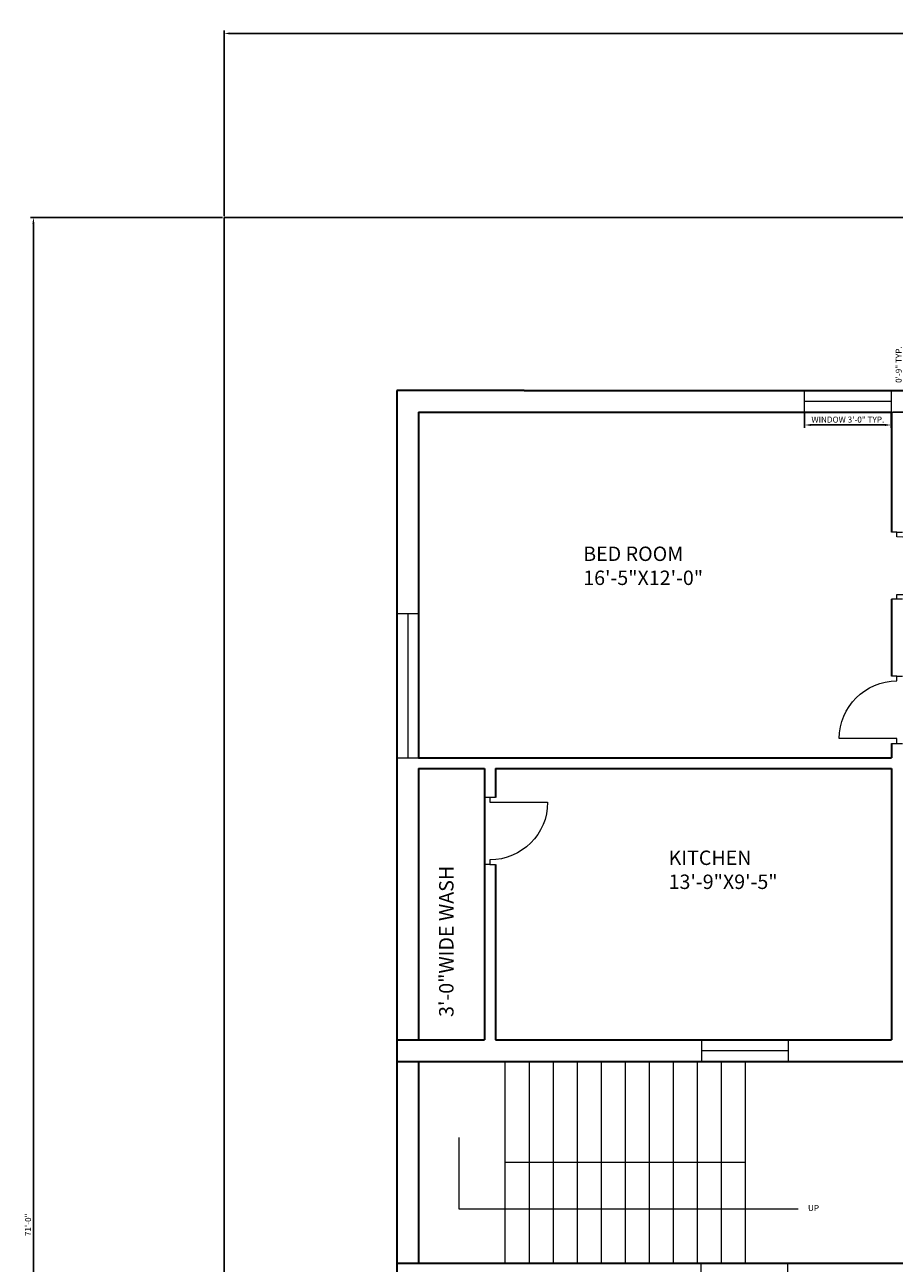
# Model space of a CAD drawing. Units: inches. Extents: x 3257 to 4085, y -12 to 956.
# Tile 4 of 6: x 3257 to 3619, y 441 to 956. Entities that reach past the tile are written whole.
import ezdxf

# ---------------------------------------------------------------- set-up
doc = ezdxf.new("R2010")
doc.units = ezdxf.units.IN
for name, color, linetype, lineweight in [('A-ANNO-DIMS', 2, 'Continuous', 18), ('A-ANNO-TEXT', 7, 'Continuous', 18), ('A-AREA-IDEN', 7, 'Continuous', 18), ('A-DOOR', 3, 'Continuous', 18), ('A-FLOR-STRS', 7, 'Continuous', 18), ('A-GLAZ', 4, 'Continuous', 18), ('A-WALL', 7, 'Continuous', 35), ('C-PROP', 6, 'Continuous', 25)]:
    doc.layers.add(name, color=color, linetype=linetype, lineweight=lineweight)
doc.styles.get("Standard").update_dxf_attribs({"font": 'arial.ttf'})
doc.dimstyles.new('ISO-25', dxfattribs={"dimtxt": 2.5, "dimasz": 2.5, "dimexe": 1.25, "dimexo": 0.625, "dimtad": 1, "dimdec": 0, "dimlunit": 3, "dimtxsty": 'Standard', "dimcen": 2.5, "dimadec": 0, "dimazin": 0, "dimtfac": 1, "dimtdec": 0, "dimtmove": 0, "dimatfit": 3, "dimfxl": 1, "dimarcsym": 0})

# ---------------------------------------------------------------- blocks, each defined once
blk = doc.blocks.new('*D1')
at = {"layer": 'A-ANNO-DIMS', "color": 0, "lineweight": -2, "transparency": 16777216}
for p, q in [((3339.97, 876.63), (3339.97, 953.92)), ((3342.47, 952.67), (4033.97, 952.67)), ((4036.47, 876.63), (4036.47, 953.92))]:
    blk.add_line(p, q, dxfattribs=at)
at = {"layer": 'A-ANNO-DIMS', "color": 0, "transparency": 16777216}
for points in [[(3342.47, 953.09), (3342.47, 952.25), (3339.97, 952.67)], [(4033.97, 953.09), (4033.97, 952.25), (4036.47, 952.67)]]:
    blk.add_solid(points, dxfattribs=at)
at = {"layer": 'Defpoints', "color": 0, "transparency": 16777216}
for p in [(4036.47, 952.67), (3339.97, 876), (4036.47, 876)]:
    blk.add_point(p, dxfattribs=at)
at = {"layer": 'A-ANNO-DIMS', "color": 0, "transparency": 16777216, "insert": (3688.22, 954.57), "char_height": 2.5, "attachment_point": 5}
blk.add_mtext('56\'-0"', dxfattribs=at)
blk = doc.blocks.new('*D2')
at = {"layer": 'A-ANNO-DIMS', "color": 0, "lineweight": -2, "transparency": 16777216}
for p, q in [((3339.34, 876), (3259.3, 876)), ((3260.55, 873.5), (3260.55, 39.5)), ((3339.34, 37), (3259.3, 37))]:
    blk.add_line(p, q, dxfattribs=at)
at = {"layer": 'A-ANNO-DIMS', "color": 0, "transparency": 16777216}
for points in [[(3260.13, 873.5), (3260.97, 873.5), (3260.55, 876)], [(3260.13, 39.5), (3260.97, 39.5), (3260.55, 37)]]:
    blk.add_solid(points, dxfattribs=at)
at = {"layer": 'Defpoints', "color": 0, "transparency": 16777216}
for p in [(3339.97, 876), (3260.55, 37), (3339.97, 37)]:
    blk.add_point(p, dxfattribs=at)
at = {"layer": 'A-ANNO-DIMS', "color": 0, "transparency": 16777216, "insert": (3258.65, 456.5), "char_height": 2.5, "attachment_point": 5, "rotation": 90}
blk.add_mtext('71\'-0"', dxfattribs=at)
blk = doc.blocks.new('DOOR-SGL-24IN')
for p, q in [((2.25, 28), (0, 28)), ((2.25, 26), (2.25, 28)), ((2.25, 28), (4.5, 28)), ((2.25, 0), (2.25, 2)), ((2.25, 2), (26.25, 2)), ((4.5, 0), (0, 0))]:
    blk.add_line(p, q)
blk.add_arc((2.25, 2), 24, 0, 90)
blk = doc.blocks.new('WIN-36IN')
for p, q in [((0, 9), (36, 9)), ((0, 0), (0, 9)), ((36, 9), (36, 0)), ((0, 4.5), (36, 4.5)), ((36, 0), (0, 0))]:
    blk.add_line(p, q)
blk = doc.blocks.new('WIN-60IN')
for p, q in [((0, 60), (0, 0)), ((9, 60), (0, 60)), ((4.5, 60), (4.5, 0)), ((9, 0), (9, 60)), ((0, 0), (9, 0))]:
    blk.add_line(p, q)
blk = doc.blocks.new('*D12')
at = {"layer": 'A-ANNO-DIMS', "color": 0, "lineweight": -2, "transparency": 16777216}
for p, q in [((3581.77, 794.38), (3581.77, 788.35)), ((3617.77, 794.38), (3617.77, 788.35)), ((3584.27, 789.6), (3615.27, 789.6))]:
    blk.add_line(p, q, dxfattribs=at)
at = {"layer": 'A-ANNO-DIMS', "color": 0, "transparency": 16777216}
for points in [[(3584.27, 790.02), (3584.27, 789.19), (3581.77, 789.6)], [(3615.27, 790.02), (3615.27, 789.19), (3617.77, 789.6)]]:
    blk.add_solid(points, dxfattribs=at)
at = {"layer": 'Defpoints', "color": 0, "transparency": 16777216}
for p in [(3581.77, 795), (3617.77, 795), (3617.77, 789.6)]:
    blk.add_point(p, dxfattribs=at)
at = {"layer": 'A-ANNO-DIMS', "color": 0, "transparency": 16777216, "insert": (3599.77, 791.52), "char_height": 2.5, "attachment_point": 5}
blk.add_mtext('WINDOW 3\'-0" TYP.', dxfattribs=at)
blk = doc.blocks.new('*D13')
at = {"layer": 'A-ANNO-DIMS', "color": 0, "lineweight": -2, "transparency": 16777216}
for p, q in [((3623.17, 804), (3623.17, 822.99)), ((3618.39, 804), (3624.42, 804)), ((3623.17, 797.5), (3623.17, 801.5)), ((3618.39, 795), (3624.42, 795))]:
    blk.add_line(p, q, dxfattribs=at)
at = {"layer": 'A-ANNO-DIMS', "color": 0, "transparency": 16777216}
for points in [[(3622.75, 801.5), (3623.58, 801.5), (3623.17, 804)], [(3622.75, 797.5), (3623.58, 797.5), (3623.17, 795)]]:
    blk.add_solid(points, dxfattribs=at)
at = {"layer": 'Defpoints', "color": 0, "transparency": 16777216}
for p in [(3617.77, 804), (3623.17, 804), (3617.77, 795)]:
    blk.add_point(p, dxfattribs=at)
at = {"layer": 'A-ANNO-DIMS', "color": 0, "transparency": 16777216, "insert": (3621.26, 814.75), "char_height": 2.5, "attachment_point": 5, "rotation": 90}
blk.add_mtext('0\'-9" TYP.', dxfattribs=at)

msp = doc.modelspace()

# ---------------------------------------------------------------- linework, layer by layer
at = {"layer": 'A-FLOR-STRS'}
for p, q in [((3456.97, 524.5), (3456.97, 440.5)), ((3466.97, 524.5), (3466.97, 440.5)), ((3476.97, 524.5), (3476.97, 440.5)), ((3486.97, 524.5), (3486.97, 440.5)), ((3496.97, 524.5), (3496.97, 440.5)), ((3506.97, 524.5), (3506.97, 440.5)), ((3516.97, 524.5), (3516.97, 440.5)), ((3526.97, 524.5), (3526.97, 440.5)), ((3536.97, 524.5), (3536.97, 440.5)), ((3546.97, 524.5), (3546.97, 440.5)), ((3556.97, 524.5), (3556.97, 440.5)), ((3437.81, 492.9), (3437.81, 463.21)), ((3556.97, 482.5), (3456.97, 482.5)), ((3437.81, 463.21), (3579.08, 463.21))]:
    msp.add_line(p, q, dxfattribs=at)
at = {"layer": 'A-WALL'}
for p, q in [((3464.97, 804), (3411.97, 804)), ((3411.97, 804), (3411.97, 795)), ((3464.97, 804), (3928.47, 804)), ((3411.97, 795), (3411.97, 745)), ((3420.97, 795), (3420.97, 745)), ((3420.97, 795), (3473.97, 795)), ((3473.97, 795), (3617.97, 795)), ((3617.97, 795), (3617.97, 745)), ((3411.97, 745), (3411.97, 157)), ((3420.97, 745), (3420.97, 651)), ((3617.97, 717), (3617.97, 685)), ((3617.97, 657), (3617.97, 651)), ((3420.97, 651), (3617.97, 651)), ((3420.97, 646.5), (3448.47, 646.5)), ((3420.97, 646.5), (3420.97, 533.5)), ((3448.47, 646.5), (3448.47, 533.5)), ((3452.97, 646.5), (3452.97, 634.5)), ((3452.97, 646.5), (3617.97, 646.5)), ((3452.97, 646.5), (3452.97, 634.5)), ((3617.97, 646.5), (3617.97, 533.5)), ((3452.97, 606.5), (3452.97, 533.5)), ((3411.97, 533.5), (3448.47, 533.5)), ((3452.97, 533.5), (3617.97, 533.5)), ((3411.97, 524.5), (3886.47, 524.5)), ((3420.97, 524.5), (3420.97, 440.5)), ((3411.97, 440.5), (3886.47, 440.5))]:
    msp.add_line(p, q, dxfattribs=at)
at = {"layer": 'C-PROP'}
for p, q in [((3464.97, 876), (3339.97, 876)), ((3339.97, 795), (3339.97, 876)), ((3464.97, 876), (3928.47, 876)), ((3339.97, 795), (3339.97, 745)), ((3339.97, 745), (3339.97, 37))]:
    msp.add_line(p, q, dxfattribs=at)

# ---------------------------------------------------------------- block references
at = {"layer": 'A-DOOR'}
msp.add_blockref('DOOR-SGL-24IN', (3617.97, 717), dxfattribs=at)
at = {"layer": 'A-DOOR', "extrusion": (0, 0, -1), "zscale": -1}
msp.add_blockref('DOOR-SGL-24IN', (-3622.47, 657), dxfattribs=at)
at = {"layer": 'A-DOOR', "extrusion": (0, 0, -1), "zscale": -1, "rotation": 180}
msp.add_blockref('DOOR-SGL-24IN', (-3448.47, 634.5), dxfattribs=at)
at = {"layer": 'A-GLAZ'}
for name, p in [('WIN-36IN', (3581.77, 795)), ('WIN-60IN', (3411.97, 651))]:
    msp.add_blockref(name, p, dxfattribs=at)
at = {"layer": 'A-GLAZ', "rotation": 180}
for p in [(3574.97, 533.5), (3574.64, 440.5)]:
    msp.add_blockref('WIN-36IN', p, dxfattribs=at)

# ---------------------------------------------------------------- texts
at = {"layer": 'A-ANNO-TEXT', "insert": (3583.16, 464.74), "char_height": 2.5, "attachment_point": 1}
msp.add_mtext('UP', dxfattribs=at)
at = {"layer": 'A-AREA-IDEN', "char_height": 6, "attachment_point": 1}
for s, insert in [('BED ROOM\\P16\'-5"X12\'-0"', (3489.55, 738.96)), ('KITCHEN\\P13\'-9"X9\'-5"', (3525.12, 612.36))]:
    msp.add_mtext(s, dxfattribs=dict(at, insert=insert))
at = {"layer": 'A-AREA-IDEN', "insert": (3429.53, 543.06), "char_height": 6, "attachment_point": 1, "rotation": 90}
msp.add_mtext('3\'-0"WIDE WASH', dxfattribs=at)

# ---------------------------------------------------------------- dimensions: what is measured, and where the dimension line sits
at = {"layer": 'A-ANNO-DIMS'}
for base, p1, p2, text, override, picture, middle in [((4036.47, 952.67), (3339.97, 876), (4036.47, 876), '56\'-0"', {"dimclrd": 0, "dimclre": 0, "dimclrt": 0}, '*D1', (3688.22, 954.57)), ((3617.77, 789.6), (3581.77, 795), (3617.77, 795), 'WINDOW <> TYP.', {"dimdec": 1, "dimlfac": 1, "dimrnd": 0, "dimzin": 1, "dimdsep": 46, "dimlunit": 4, "dimfrac": 2}, '*D12', (3599.77, 791.52))]:
    dim = msp.add_linear_dim(base=base, p1=p1, p2=p2, text=text, dimstyle='ISO-25', override=override, dxfattribs=at)
    dim.commit()
    dim.dimension.update_dxf_attribs({"geometry": picture, "text_midpoint": middle})
for base, p1, p2, text, override, picture, middle in [((3260.55, 37), (3339.97, 876), (3339.97, 37), '71\'-0"', {"dimclrd": 0, "dimclre": 0, "dimclrt": 0}, '*D2', (3258.65, 456.5)), ((3623.17, 804), (3617.77, 795), (3617.77, 804), '<> TYP.', {"dimdec": 1, "dimlfac": 1, "dimrnd": 0, "dimzin": 1, "dimdsep": 46, "dimlunit": 4, "dimfrac": 2}, '*D13', (3621.26, 814.75))]:
    dim = msp.add_linear_dim(base=base, p1=p1, p2=p2, angle=90, text=text, dimstyle='ISO-25', override=override, dxfattribs=at)
    dim.commit()
    dim.dimension.update_dxf_attribs({"geometry": picture, "text_midpoint": middle})

doc.saveas('drawing.dxf')
